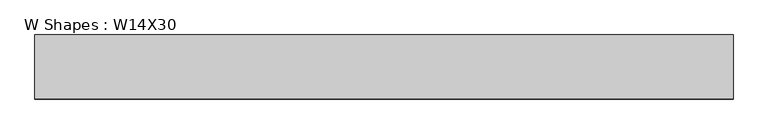
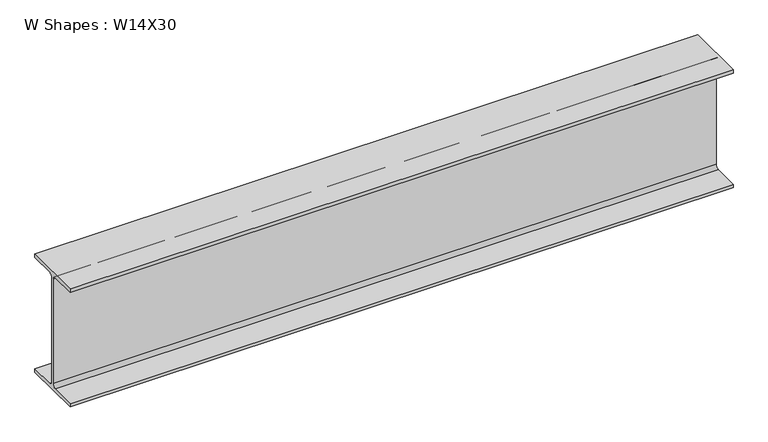
"""IFC4 building model written with IfcOpenShell, lengths in millimetres: beam geometry, W Shapes : W14X30."""

from ifc_helpers import new_model, si_unit, point, frame, frame_2d, origin, place, context, project, spatial, polyline, circle_curve, trimmed, segment, composite_curve, outline, extrude, source, transform, mapped, element, save


def w_shapes_w14x30_72b19b1b(model_context):
    return source(origin(), model_context, "Body", "SweptSolid", [
        extrude(outline(composite_curve([segment(polyline([(85.471, -165.481), (85.471, -175.26), (-85.471, -175.26), (-85.471, -165.481), (-13.589, -165.481)]), True, "CONTINUOUS"), segment(trimmed(circle_curve(frame_2d((-13.589, -155.321)), 10.16), [point((-13.589, -165.481))], [point((-3.429, -155.321))], True, "CARTESIAN"), True, "CONTINUOUS"), segment(polyline([(-3.429, -155.321), (-3.429, 155.321)]), True, "CONTINUOUS"), segment(trimmed(circle_curve(frame_2d((-13.589, 155.321)), 10.16), [point((-3.429, 155.321))], [point((-13.589, 165.481))], True, "CARTESIAN"), True, "CONTINUOUS"), segment(polyline([(-13.589, 165.481), (-85.471, 165.481), (-85.471, 175.26), (85.471, 175.26), (85.471, 165.481), (13.589, 165.481)]), True, "CONTINUOUS"), segment(trimmed(circle_curve(frame_2d((13.589, 155.321)), 10.16), [point((13.589, 165.481))], [point((3.429, 155.321))], True, "CARTESIAN"), True, "CONTINUOUS"), segment(polyline([(3.429, 155.321), (3.429, -155.321)]), True, "CONTINUOUS"), segment(trimmed(circle_curve(frame_2d((13.589, -155.321)), 10.16), [point((3.429, -155.321))], [point((13.589, -165.481))], True, "CARTESIAN"), True, "CONTINUOUS"), segment(polyline([(13.589, -165.481), (85.471, -165.481)]), True, "CONTINUOUS")], self_intersect=False)), frame((-955.04, 0.0, 0.0), z_axis=(1.0, 0.0, 0.0), x_axis=(0.0, 1.0, 0.0)), (0.0, 0.0, 1.0), 1862.2095299),
    ])


if __name__ == "__main__":
    model = new_model("IFC4")
    model_context = context("Model", 3, world=origin())
    ifc_project = project(units=[si_unit("LENGTHUNIT", "METRE", prefix="MILLI")], contexts=[model_context])
    site = spatial("IfcSite", under=ifc_project)
    building = spatial("IfcBuilding", under=site)
    placement = place(None, origin())
    w_shapes_w14x30_shape = w_shapes_w14x30_72b19b1b(model_context)
    element("IfcBeam", 1, ObjectType="W Shapes : W14X30", at=placement, inside=building, context=model_context, shape_type="MappedRepresentation", body=[
        mapped(w_shapes_w14x30_shape, transform((0.0, 0.0, 0.0), x_axis=(1.0, 0.0, 0.0), y_axis=(0.0, 1.0, 0.0), z_axis=(0.0, 0.0, 1.0))),
    ])
    save(model, "model.ifc")

# Revit data of these elements
# Type "W Shapes : W14X30"
#   Section Name Key = "W14X30"
#   Width = 6.730"
#   Web Thickness = 0.270"
#   Web Fillet = 0.400"
#   Warping Constant = 887.00 in⁶
#   Torsional Moment of Inertia = 0.38 in⁴
#   Section Area = 8.85 in²
#   Plastic Modulus weak axis = 8.99 in³
#   Plastic Modulus strong axis = 47.30 in³
#   Perimeter = 4.441 ft²/ft
#   Nominal Weight = 30.00 lbf/ft
#   Moment of Inertia weak axis = 19.60 in⁴
#   Moment of Inertia strong axis = 291.00 in⁴
#   Height = 13.800"
#   Flange Thickness = 0.385"
#   Elastic Modulus weak axis = 5.82 in³
#   Elastic Modulus strong axis = 42.00 in³
#   Clear Web Height = 0' - 11 5/8"
#   Centroid Vertical = 6.900"
#   Centroid Horizontal = 3.365"
#   Bolt Spacing = 0' - 3 1/2"
#   Length [instance default] = 1524 mm
#   Structural Material [instance default] = Steel ASTM A992
#   Principal Axes Angle = 0
# Element 1 (IfcBeam, "W Shapes : W14X30")
#   Length = 2286 mm
#   Materials on its faces: "Steel ASTM A992"
# Materials
#   "Steel ASTM A992": class "Metal", colour RGB 199 199 199, transparency 0, Description = "Structural steel 50ksi", Cost = 0
